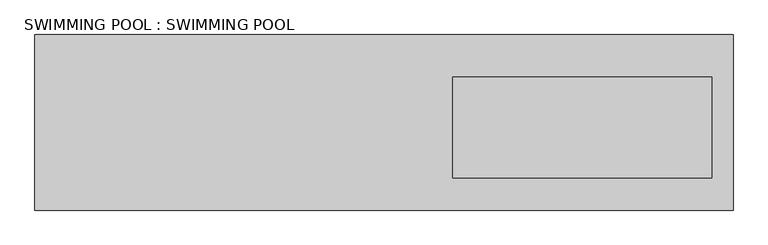
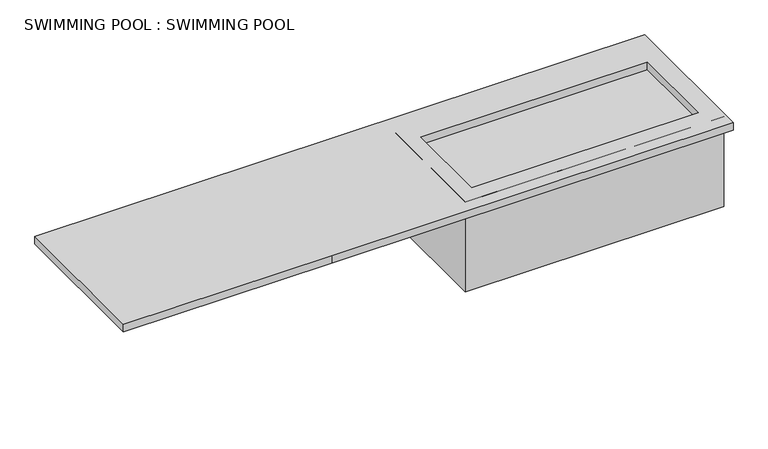
"""IFC4 building model written with IfcOpenShell, lengths in millimetres: proxy geometry, SWIMMING POOL : SWIMMING POOL."""

from ifc_helpers import new_model, si_unit, frame, origin, place, context, project, spatial, polyline, outline, extrude, faceted_brep, source, transform, mapped, element, save


def swimming_pool_swimming_pool_f5703ba1(model_context):
    return source(origin(), model_context, "Body", "SolidModel", [
        extrude(outline(polyline([(-11510.4862037, -7514.2678797), (-15493.3362671, -7514.2678797), (-15493.3362671, -4589.1704973), (-3864.1794909, -4589.1704973), (-3864.1794909, -7514.2678797), (-11510.4862037, -7514.2678797)]), holes=[polyline([(-4219.7794909, -5292.6831876), (-8537.7967506, -5292.6831876), (-8537.7967506, -6980.8678797), (-4219.7794909, -6980.8678797), (-4219.7794909, -5292.6831876)])]), frame((0.0, 0.0, -152.4), z_axis=(0.0, 0.0, 1.0), x_axis=(1.0, 0.0, 0.0)), (0.0, 0.0, 1.0), 152.4),
        faceted_brep([(-3914.9794909, -4987.8831876, -1808.6014922), (-3914.9794909, -7285.6678797, -1808.6014922), (-8842.5967506, -7285.6678797, -1808.6014922), (-8842.5967506, -4987.8831876, -1808.6014922), (-3914.9794909, -4987.8831876, 0.0), (-8842.5967506, -4987.8831876, 0.0), (-8842.5967506, -7285.6678797, 0.0), (-3914.9794909, -7285.6678797, 0.0), (-4219.7794909, -5292.6831876, 0.0), (-4219.7794909, -6980.8678797, 0.0), (-8537.7967506, -6980.8678797, 0.0), (-8537.7967506, -5292.6831876, 0.0), (-4219.7794909, -5292.6831876, -152.4), (-8537.7967506, -5292.6831876, -152.4), (-8537.7967506, -6980.8678797, -152.4), (-4219.7794909, -6980.8678797, -152.4)], [[[0, 1, 2, 3]], [[4, 5, 6, 7], [8, 9, 10, 11]], [[0, 3, 5, 4]], [[3, 2, 6, 5]], [[2, 1, 7, 6]], [[1, 0, 4, 7]], [[12, 13, 14, 15]], [[12, 15, 9, 8]], [[15, 14, 10, 9]], [[14, 13, 11, 10]], [[13, 12, 8, 11]]]),
    ])


if __name__ == "__main__":
    model = new_model("IFC4")
    model_context = context("Model", 3, world=origin())
    ifc_project = project(units=[si_unit("LENGTHUNIT", "METRE", prefix="MILLI")], contexts=[model_context])
    site = spatial("IfcSite", under=ifc_project)
    building = spatial("IfcBuilding", under=site)
    placement = place(None, origin())
    swimming_pool_swimming_pool_shape = swimming_pool_swimming_pool_f5703ba1(model_context)
    element("IfcBuildingElementProxy", 1, Name="SWIMMING POOL : SWIMMING POOL", ObjectType="SWIMMING POOL : SWIMMING POOL", at=placement, inside=building, context=model_context, shape_type="MappedRepresentation", body=[
        mapped(swimming_pool_swimming_pool_shape, transform((0.0, 0.0, 0.0), x_axis=(1.0, 0.0, 0.0), y_axis=(0.0, 1.0, 0.0), z_axis=(0.0, 0.0, 1.0))),
    ])
    save(model, "model.ifc")

# Revit data of these elements
# Element 1 (IfcBuildingElementProxy, "SWIMMING POOL : SWIMMING POOL")
#   Materials on its faces: "Water", "SWIMMING POOL", "WALL 3"
# Materials
#   "Water": class "Liquid", colour RGB 108 195 217, transparency 0, Description = "Water", Cost = 0
#   "SWIMMING POOL": class "Generic", colour RGB 120 120 120, transparency 0, Cost = 0
#   "WALL 3": class "Generic", colour RGB 120 120 120, transparency 0, Cost = 0
